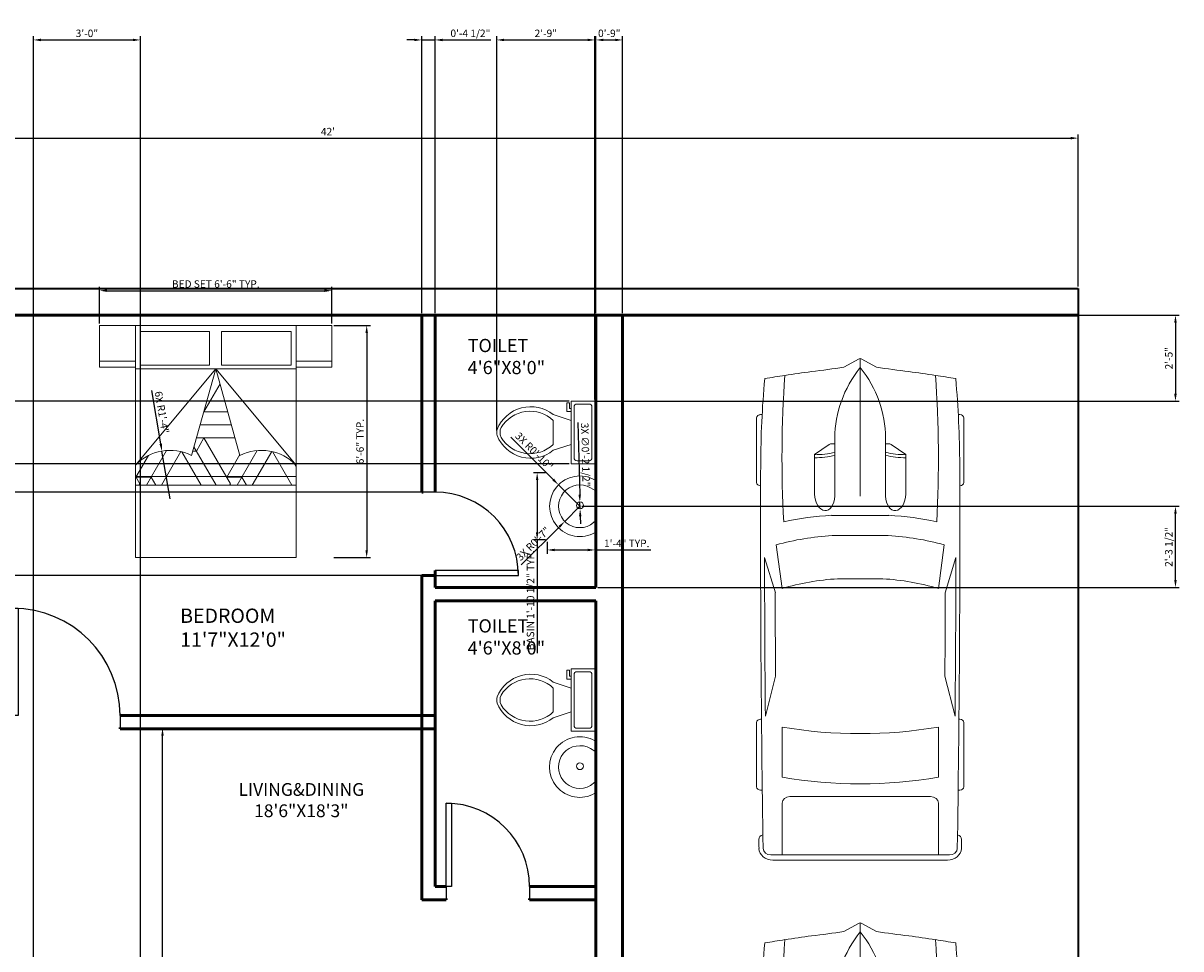
# Model space of a CAD drawing. Units: inches. Extents: x 1455 to 2044, y 1728 to 2439.
# Tile 4 of 4: x 1655 to 2044, y 2128 to 2439. Entities that reach past the tile are written whole.
import ezdxf

# ---------------------------------------------------------------- set-up
doc = ezdxf.new("R2010")
doc.units = ezdxf.units.IN
for name, color, linetype, lineweight in [('A-ANNO-DIMS', 2, 'Continuous', 18), ('A-AREA-IDEN', 7, 'Continuous', 25), ('A-DOOR', 4, 'Continuous', 25), ('A-FLOR-FIXT', 9, 'Continuous', 18), ('A-FURN', 8, 'Continuous', 18), ('A-WALL', 7, 'Continuous', 50), ('C-PRKG-VEHI', 8, 'Continuous', 13), ('C-PROP', 7, 'Continuous', 35)]:
    doc.layers.add(name, color=color, linetype=linetype, lineweight=lineweight)
doc.styles.get("Standard").update_dxf_attribs({"font": 'arial.ttf'})
doc.dimstyles.new('ISO-25', dxfattribs={"dimtxt": 2.5, "dimasz": 2.5, "dimexe": 1.25, "dimexo": 0.625, "dimtad": 1, "dimlunit": 3, "dimtxsty": 'Standard', "dimcen": 2.5, "dimadec": 0, "dimazin": 0, "dimtfac": 1, "dimtmove": 0, "dimatfit": 3, "dimfxl": 1, "dimarcsym": 0})

# ---------------------------------------------------------------- blocks, each defined once
blk = doc.blocks.new('*U7')
for p, q in [((0, 0), (0, -4)), ((36, 0), (36, -4))]:
    blk.add_line(p, q)
blk.add_lwpolyline([(0, 0), (0, 36), (1.75, 36), (1.75, 0)], close=True)
blk.add_arc((0, 0), 36, 0, 90)
blk = doc.blocks.new('*U4')
for p, q in [((-28, 0), (-28, -4)), ((0, 0), (0, -4))]:
    blk.add_line(p, q)
blk.add_lwpolyline([(0, 0), (0, 28), (-1.75, 28), (-1.75, 0)], close=True)
blk.add_arc((0, 0), 28, 90, 180)
blk = doc.blocks.new('*U5')
for p, q in [((0, 0), (0, -4)), ((28, 0), (28, -4))]:
    blk.add_line(p, q)
blk.add_lwpolyline([(0, 0), (0, 28), (1.75, 28), (1.75, 0)], close=True)
blk.add_arc((0, 0), 28, 0, 90)
blk = doc.blocks.new('*U2')
for p, q in [((9.5, -6), (9.5, -2)), ((-10, -8.5), (-8, -8.5)), ((-10, -9.5), (-10, -8.5)), ((-7, -9.5), (-10, -9.5)), ((-8, -8.5), (-8, -8)), ((-7, -8), (-7, -9.5)), ((-4, -8), (-6, -14)), ((4, -8), (6, -14)), ((4, -14), (-4, -14))]:
    blk.add_line(p, q)
blk.add_lwpolyline([(10.5, -8), (10.5, 0), (-10.5, 0), (-10.5, -8)], close=True)
for points in [[(-9.5, -2), (-9.5, -6)], [(8.5, -1), (-8.5, -1)], [(-8.5, -7), (8.5, -7)]]:
    blk.add_lwpolyline(points)
for centre, radius, start, end in [((-8.62, -1.88), 0.884, 81.8699, 188.1301), ((8.62, -1.88), 0.884, 351.8699, 98.1301), ((-8.62, -6.12), 0.884, 171.8699, 278.1301), ((8.62, -6.12), 0.884, 261.8699, 8.1301), ((3.52, -21.58), 12.17, 141.4691, 247.9714), ((4.2, -21.82), 11.33, 136.3677, 238.9468), ((-3.52, -21.58), 12.17, 292.0284, 38.5307), ((-4.2, -21.82), 11.33, 301.053, 43.6321), ((0, -27.88), 4, 245.7318, 294.2682), ((0, -29), 4, 254.8605, 285.1395)]:
    blk.add_arc(centre, radius, start, end)
blk = doc.blocks.new('*D17')
at = {"layer": 'A-ANNO-DIMS', "color": 0, "lineweight": -2, "transparency": 16777216}
for p, q in [((1505.58, 2350.2), (1505.58, 2401.3)), ((1508.08, 2400.05), (2007.08, 2400.05)), ((2009.58, 2350.2), (2009.58, 2401.3))]:
    blk.add_line(p, q, dxfattribs=at)
at = {"layer": 'A-ANNO-DIMS', "color": 0, "transparency": 16777216}
for points in [[(1508.08, 2400.47), (1508.08, 2399.63), (1505.58, 2400.05)], [(2007.08, 2400.47), (2007.08, 2399.63), (2009.58, 2400.05)]]:
    blk.add_solid(points, dxfattribs=at)
at = {"layer": 'Defpoints', "color": 0, "transparency": 16777216}
for p in [(2009.58, 2400.05), (1505.58, 2349.58), (2009.58, 2349.58)]:
    blk.add_point(p, dxfattribs=at)
at = {"layer": 'A-ANNO-DIMS', "color": 0, "transparency": 16777216, "insert": (1757.58, 2401.93), "char_height": 2.5, "attachment_point": 5}
blk.add_mtext("42'", dxfattribs=at)
blk = doc.blocks.new('*U19')
for p, q in [((21.1, 37.41), (21.1, 36.83)), ((46.55, 38.89), (22.35, 38.89)), ((47.8, 37.39), (47.8, 37.41)), ((87.99, 31.87), (74.76, 35.92)), ((134.31, 35.6), (119.29, 31.78)), ((135.45, 37.07), (135.45, 37.41)), ((136.7, 38.89), (160.9, 38.89)), ((162.15, 37.41), (162.15, 36.77)), ((70.03, 31.54), (86.41, 29.35)), ((186.47, -33.5), (186.47, 33.5)), ((188.4, -32.76), (188.4, 32.76)), ((138.42, 29.35), (157.25, 29.35)), ((164.52, 26.39), (164.52, -26.39)), ((186.47, 29.35), (167.01, 29.35)), ((32.27, 11.63), (36.13, 17.17)), ((36.13, 17.17), (50.94, 17.17)), ((29.77, 9.51), (51.68, 9.51)), ((32.12, 9.51), (32.12, 11.15)), ((58.92, -10.77), (58.92, 10.77)), ((66.55, -10.53), (66.55, 10.53)), ((186.47, -10.53), (186.47, 10.53)), ((3.27, 6.13), (0.1, 0.41)), ((82.74, 8.5), (82.74, -8.5)), ((0, 0), (51.68, 0)), ((0.1, -0.41), (3.27, -6.13)), ((29.77, -9.51), (51.68, -9.51)), ((32.12, -9.51), (32.12, -11.15)), ((32.27, -11.63), (36.13, -17.17)), ((36.13, -17.17), (50.94, -17.17)), ((86.41, -29.35), (70.03, -31.54)), ((157.25, -29.35), (138.42, -29.35)), ((167.01, -29.35), (186.47, -29.35)), ((87.99, -31.87), (74.76, -35.92)), ((134.31, -35.6), (119.29, -31.78)), ((21.1, -37.41), (21.1, -36.83)), ((46.55, -38.89), (22.35, -38.89)), ((47.8, -37.39), (47.8, -37.41)), ((135.45, -37.07), (135.45, -37.41)), ((136.7, -38.89), (160.9, -38.89)), ((162.15, -37.41), (162.15, -36.77))]:
    blk.add_line(p, q)
for centre, major_axis, ratio, start_param, end_param in [((266.03, -27.52), (0, 313.31), 0.842304, 1.367076, 1.39176), ((41.19, -490.86), (0, 528.23), 0.842304, 0.00281, 0.075598), ((22.35, 37.41), (0, -1.48), 0.842304, 3.141593, 4.712389), ((64.48, -10555.62), (0, 10593.03), 0.842304, -0.013397, 0.002797), ((46.55, 37.41), (0, 1.48), 0.842304, -1.570796, 0), ((64.48, -10555.62), (0, -10591.55), 0.842304, 3.133765, 3.140441), ((136.7, 37.41), (0, -1.48), 0.842304, 3.141593, 4.712389), ((160.9, 37.41), (0, 1.48), 0.842304, -1.570796, 0), ((180.63, 35.84), (0, 2.22), 0.842304, -0.013017, 1.249894), ((64.48, -10556.36), (0, 10595.31), 0.842304, -0.013397, -0.013017), ((183.98, 33.5), (0, -2.96), 0.842304, 1.570796, 3.128196), ((183.98, 32.76), (0, -5.25), 0.842304, 1.570796, 3.128196), ((135.29, 5.39), (0, 81.77), 0.842304, 1.245306, 1.50788), ((95.79, -3666.35), (0, -3698.24), 0.842304, 3.134049, 3.144098), ((259.18, -27.52), (0, -305.3), 0.842304, 4.528606, 4.561838), ((37.47, -593.96), (0, -623.33), 0.842304, 3.096046, 3.200911), ((134.4, 5.39), (0, -89.78), 0.842304, 4.449482, 4.652344), ((149.6, 2.8), (0, -79.58), 0.842304, 4.372215, 4.640744), ((17.08, 0), (0, 147.02), 0.842304, 4.511394, 4.913384), ((35.91, 0), (0, 147.02), 0.842304, 4.511394, 4.913384), ((167.01, 26.39), (0, 2.96), 0.842304, 0, 1.570796), ((-204.49, 52.4), (0, -250.96), 0.842304, 1.385369, 1.434372), ((13.04, 17.01), (0, 27.42), 0.842304, 4.435146, 4.718221), ((14.2, 17.01), (0, 27.42), 0.842304, 4.435146, 4.718221), ((50.79, 13.34), (6.34, -0.36), 0.603834, -1.395552, 1.581315), ((29.77, -46.66), (0, 56.17), 0.842304, 0, 0.590319), ((32.75, 11.15), (0, 0.74), 0.842304, 0.879714, 1.570796), ((0.62, 0), (0, -0.74), 0.842304, 4.131459, 5.293319), ((29.77, 46.66), (0, 56.17), 0.842304, 2.551274, 3.141593), ((-204.49, -52.4), (0, 250.96), 0.842304, -1.434372, -1.385369), ((149.6, -2.8), (0, -79.58), 0.842304, -1.499151, -1.230623), ((32.75, -11.15), (0, -0.74), 0.842304, 4.712389, 5.403472), ((13.04, -17.01), (0, -27.42), 0.842304, 1.564964, 1.848039), ((14.2, -17.01), (0, -27.42), 0.842304, 1.564964, 1.848039), ((134.4, -5.39), (0, -89.78), 0.842304, -1.510751, -1.307889), ((135.29, -5.39), (0, -81.77), 0.842304, -1.50788, -1.245306), ((259.18, 27.52), (0, 305.3), 0.842304, 1.721348, 1.754579), ((266.03, 27.52), (0, 313.31), 0.842304, 1.749832, 1.774517), ((37.47, 593.96), (0, -623.33), 0.842304, -0.059319, 0.045547), ((167.01, -26.39), (0, -2.96), 0.842304, 4.712389, 6.283185), ((95.79, 3666.35), (0, -3698.24), 0.842304, -0.002505, 0.007544), ((183.98, -33.5), (0, 2.96), 0.842304, 3.15499, 4.712389), ((183.98, -32.76), (0, -5.25), 0.842304, 0.013397, 1.570796), ((41.19, 490.86), (0, -528.23), 0.842304, -0.075598, -0.00281), ((22.35, -37.41), (0, 1.48), 0.842304, 1.570796, 3.141593), ((64.48, 10555.62), (0, 10593.03), 0.842304, 3.138796, 3.15499), ((46.55, -37.41), (0, -1.48), 0.842304, 0, 1.570796), ((64.48, 10555.62), (0, -10591.55), 0.842304, 0.001152, 0.007828), ((136.7, -37.41), (0, -1.48), 0.842304, -1.570796, 0), ((160.9, -37.41), (0, 1.48), 0.842304, 3.141593, 4.712389), ((180.63, -35.84), (0, -2.22), 0.842304, -1.249894, 0.013017), ((64.48, 10556.36), (0, 10595.31), 0.842304, 3.15461, 3.15499)]:
    blk.add_ellipse(centre, major_axis=major_axis, ratio=ratio, start_param=start_param, end_param=end_param)
at = {"extrusion": (0, 0, -1)}
blk.add_ellipse((50.79, -13.34), major_axis=(6.34, 0.36), ratio=0.603834, start_param=-1.395552, end_param=1.581315, dxfattribs=at)
blk = doc.blocks.new('*D20')
at = {"layer": 'A-ANNO-DIMS', "color": 0, "lineweight": -2, "transparency": 16777216}
for p, q in [((1702.63, 2201.77), (1703.25, 2201.77)), ((1702, 1985.27), (1702, 2199.27)), ((1702.63, 1982.77), (1703.25, 1982.77))]:
    blk.add_line(p, q, dxfattribs=at)
at = {"layer": 'A-ANNO-DIMS', "color": 0, "transparency": 16777216}
for points in [[(1701.59, 2199.27), (1702.42, 2199.27), (1702, 2201.77)], [(1701.59, 1985.27), (1702.42, 1985.27), (1702, 1982.77)]]:
    blk.add_solid(points, dxfattribs=at)
at = {"layer": 'Defpoints', "color": 0, "transparency": 16777216}
for p in [(1702, 2201.77), (1702, 2201.77), (1702, 1982.77)]:
    blk.add_point(p, dxfattribs=at)
at = {"layer": 'A-ANNO-DIMS', "color": 0, "transparency": 16777216, "insert": (1700.1, 2092.27), "char_height": 2.5, "attachment_point": 5, "rotation": 90}
blk.add_mtext('18\'-3"', dxfattribs=at)
blk = doc.blocks.new('BED-DOUBLE-WITH-NIGHTSTANDS')
h = blk.add_hatch()
h.set_pattern_fill('ESCHER', color=256, angle=-270)
h.set_pattern_definition([(150, (2210.078, -2055.985), (7e-09, -30.48), [27.94, -2.54]), (270, (2210.078, -2055.985), (26.39645, 15.24), [27.94, -2.54]), (30, (2210.078, -2055.985), (7e-09, 30.48), [27.94, -2.54]), (150, (2210.078, -2053.445), (7e-09, -30.48), [5.08, -25.4]), (30, (2210.078, -2053.445), (7e-09, 30.48), [5.08, -25.4]), (150, (2207.88, -2057.255), (7e-09, -30.48), [5.08, -25.4]), (270, (2207.88, -2057.255), (26.39645, 15.24), [5.08, -25.4]), (30, (2212.278, -2057.255), (7e-09, 30.48), [5.08, -25.4]), (270, (2212.278, -2057.255), (26.39645, 15.24), [5.08, -25.4]), (150, (2210.078, -2066.145), (7e-09, -30.48), [5.08, -25.4]), (30, (2210.078, -2066.145), (7e-09, 30.48), [5.08, -25.4]), (150, (2218.877, -2050.905), (7e-09, -30.48), [5.08, -25.4]), (270, (2218.877, -2050.905), (26.39645, 15.24), [5.08, -25.4]), (30, (2201.28, -2050.905), (7e-09, 30.48), [5.08, -25.4]), (270, (2201.28, -2050.905), (26.39645, 15.24), [5.08, -25.4]), (90, (2205.68, -2050.905), (-26.39645, -15.24), [17.78, -12.7]), (90, (2214.478, -2050.905), (-26.39645, -15.24), [17.78, -12.7]), (210, (2203.48, -2054.715), (-7e-09, -30.48), [17.78, -12.7]), (210, (2207.88, -2062.335), (-7e-09, -30.48), [17.78, -12.7]), (330, (2212.278, -2062.335), (26.39645, 15.24), [17.78, -12.7]), (330, (2216.678, -2054.715), (26.39645, 15.24), [17.78, -12.7])])
h.paths.add_polyline_path([(-31.09, 54, 0.326433), (-34.36, 35.12), (-63.46, 27), (-34.36, 18.88, 0.326433), (-31.09, 0), (-27.21, 0), (-27.21, 54)])
h.paths.add_polyline_path([(-27.21, 54), (-27.21, 0), (-24.3, 0), (-24.3, 54)])
for p, q in [((-78, 54), (-78, 66)), ((-78, 66), (-66, 66)), ((-66, 66), (-66, 54)), ((-66, 66), (-64, 66)), ((-64, 66), (-64, 54)), ((-63.46, 0), (-63.46, 54)), ((-63.46, 27), (-31.09, 54)), ((-63.46, 27), (-34.36, 35.12)), ((-76.01, 28.95), (-64.69, 28.95)), ((-76.01, 24.95), (-64.69, 24.95)), ((-63.46, 27), (-31.09, 0)), ((-63.46, 27), (-34.36, 18.88)), ((-78, 0), (-78, -12)), ((-66, -12), (-66, 0)), ((-64, -12), (-64, 0)), ((-78, -12), (-66, -12)), ((-66, -12), (-64, -12))]:
    blk.add_line(p, q)
for points in [[(0, 0), (0, 54), (-78, 54), (-78, 0)], [(-27.21, 0), (-27.21, 54), (-24.3, 54), (-24.3, 0)]]:
    blk.add_lwpolyline(points, close=True)
for points in [[(-76.01, 28.95), (-76.01, 52.28), (-64.69, 52.28), (-64.69, 28.95)], [(-64.69, 24.95), (-64.69, 1.63), (-76.01, 1.63), (-76.01, 24.95)]]:
    blk.add_lwpolyline(points)
for centre, start, end in [((-19.81, 42.32), 134.0109, 206.3245), ((-19.81, 11.68), 153.6755, 225.9891)]:
    blk.add_arc(centre, 16.24, start, end)
blk = doc.blocks.new('BASIN-WALL-MOUNT')
for p, q in [((-6.21, 3.6), (-5.3, 5.1)), ((6.21, 3.6), (5.05, 5.1))]:
    blk.add_line(p, q)
blk.add_circle((-0.29, 0.03), 1.16)
for radius in [10.18, 7.18]:
    blk.add_arc((0, 0), radius, 149.9376, 30.0624)
blk = doc.blocks.new('*D23')
at = {"layer": 'A-ANNO-DIMS', "color": 0, "lineweight": -2, "transparency": 16777216}
for p, q in [((1680.89, 2337.73), (1680.89, 2350.05)), ((1758.89, 2337.73), (1758.89, 2350.05)), ((1683.39, 2348.8), (1756.39, 2348.8))]:
    blk.add_line(p, q, dxfattribs=at)
at = {"layer": 'A-ANNO-DIMS', "color": 0, "transparency": 16777216}
for points in [[(1683.39, 2349.22), (1683.39, 2348.39), (1680.89, 2348.8)], [(1756.39, 2349.22), (1756.39, 2348.39), (1758.89, 2348.8)]]:
    blk.add_solid(points, dxfattribs=at)
at = {"layer": 'Defpoints', "color": 0, "transparency": 16777216}
for p in [(1758.89, 2348.8), (1680.89, 2337.1), (1758.89, 2337.1)]:
    blk.add_point(p, dxfattribs=at)
at = {"layer": 'A-ANNO-DIMS', "color": 0, "transparency": 16777216, "insert": (1719.89, 2350.72), "char_height": 2.5, "attachment_point": 5}
blk.add_mtext('BED SET 6\'-6" TYP.', dxfattribs=at)
blk = doc.blocks.new('*D24')
at = {"layer": 'A-ANNO-DIMS', "color": 0, "lineweight": -2, "transparency": 16777216}
for p, q in [((1759.51, 2337.1), (1771.84, 2337.1)), ((1770.59, 2334.6), (1770.59, 2261.6)), ((1759.51, 2259.1), (1771.84, 2259.1))]:
    blk.add_line(p, q, dxfattribs=at)
at = {"layer": 'A-ANNO-DIMS', "color": 0, "transparency": 16777216}
for points in [[(1770.17, 2334.6), (1771.01, 2334.6), (1770.59, 2337.1)], [(1770.17, 2261.6), (1771.01, 2261.6), (1770.59, 2259.1)]]:
    blk.add_solid(points, dxfattribs=at)
at = {"layer": 'Defpoints', "color": 0, "transparency": 16777216}
for p in [(1758.89, 2337.1), (1758.89, 2259.1), (1770.59, 2259.1)]:
    blk.add_point(p, dxfattribs=at)
at = {"layer": 'A-ANNO-DIMS', "color": 0, "transparency": 16777216, "insert": (1768.69, 2298.1), "char_height": 2.5, "attachment_point": 5, "rotation": 90}
blk.add_mtext('6\'-6" TYP.', dxfattribs=at)
blk = doc.blocks.new('*D25')
at = {"layer": 'A-ANNO-DIMS', "color": 0, "lineweight": -2, "transparency": 16777216}
for p, q in [((1830.62, 2287.65), (1826.61, 2287.65)), ((1827.86, 2285.15), (1827.86, 2267.57)), ((1830.62, 2265.07), (1826.61, 2265.07)), ((1827.86, 2265.07), (1827.86, 2226.98))]:
    blk.add_line(p, q, dxfattribs=at)
at = {"layer": 'A-ANNO-DIMS', "color": 0, "transparency": 16777216}
for points in [[(1827.44, 2285.15), (1828.27, 2285.15), (1827.86, 2287.65)], [(1827.44, 2267.57), (1828.27, 2267.57), (1827.86, 2265.07)]]:
    blk.add_solid(points, dxfattribs=at)
at = {"layer": 'Defpoints', "color": 0, "transparency": 16777216}
for p in [(1831.24, 2287.65), (1827.86, 2265.07), (1831.24, 2265.07)]:
    blk.add_point(p, dxfattribs=at)
at = {"layer": 'A-ANNO-DIMS', "color": 0, "transparency": 16777216, "insert": (1825.94, 2244.78), "char_height": 2.5, "attachment_point": 5, "rotation": 90}
blk.add_mtext('BASIN 1\'-10 1/2" TYP.', dxfattribs=at)
blk = doc.blocks.new('*D26')
at = {"layer": 'A-ANNO-DIMS', "color": 0, "lineweight": -2, "transparency": 16777216}
for p, q in [((1831.24, 2264.45), (1831.24, 2260.44)), ((1847.32, 2264.45), (1847.32, 2260.44)), ((1833.74, 2261.69), (1844.82, 2261.69)), ((1847.32, 2261.69), (1866.07, 2261.69))]:
    blk.add_line(p, q, dxfattribs=at)
at = {"layer": 'A-ANNO-DIMS', "color": 0, "transparency": 16777216}
for points in [[(1833.74, 2262.1), (1833.74, 2261.27), (1831.24, 2261.69)], [(1844.82, 2262.1), (1844.82, 2261.27), (1847.32, 2261.69)]]:
    blk.add_solid(points, dxfattribs=at)
at = {"layer": 'Defpoints', "color": 0, "transparency": 16777216}
for p in [(1831.24, 2265.07), (1847.32, 2265.07), (1847.32, 2261.69)]:
    blk.add_point(p, dxfattribs=at)
at = {"layer": 'A-ANNO-DIMS', "color": 0, "transparency": 16777216, "insert": (1857.94, 2263.57), "char_height": 2.5, "attachment_point": 5}
blk.add_mtext('1\'-4" TYP.', dxfattribs=at)
blk = doc.blocks.new('*D32')
at = {"layer": 'A-ANNO-DIMS', "color": 0, "lineweight": -2, "transparency": 16777216}
for p, q in [((1658.63, 2034.7), (1658.63, 2434.3)), ((1661.13, 2433.05), (1692.08, 2433.05)), ((1694.58, 2034.7), (1694.58, 2434.3))]:
    blk.add_line(p, q, dxfattribs=at)
at = {"layer": 'A-ANNO-DIMS', "color": 0, "transparency": 16777216}
for points in [[(1661.13, 2433.46), (1661.13, 2432.63), (1658.63, 2433.05)], [(1692.08, 2433.46), (1692.08, 2432.63), (1694.58, 2433.05)]]:
    blk.add_solid(points, dxfattribs=at)
at = {"layer": 'Defpoints', "color": 0, "transparency": 16777216}
for p in [(1694.58, 2433.05), (1658.63, 2034.08), (1694.58, 2034.08)]:
    blk.add_point(p, dxfattribs=at)
at = {"layer": 'A-ANNO-DIMS', "color": 0, "transparency": 16777216, "insert": (1676.61, 2434.95), "char_height": 2.5, "attachment_point": 5}
blk.add_mtext('3\'-0"', dxfattribs=at)
blk = doc.blocks.new('*D37')
at = {"layer": 'A-ANNO-DIMS', "color": 0, "lineweight": -2, "transparency": 16777216}
for p, q in [((1792.95, 2281.09), (1471.63, 2281.09)), ((1472.88, 2255.58), (1472.88, 2278.59)), ((1792.95, 2253.08), (1471.63, 2253.08))]:
    blk.add_line(p, q, dxfattribs=at)
at = {"layer": 'A-ANNO-DIMS', "color": 0, "transparency": 16777216}
for points in [[(1472.46, 2278.59), (1473.3, 2278.59), (1472.88, 2281.09)], [(1472.46, 2255.58), (1473.3, 2255.58), (1472.88, 2253.08)]]:
    blk.add_solid(points, dxfattribs=at)
at = {"layer": 'Defpoints', "color": 0, "transparency": 16777216}
for p in [(1472.88, 2281.09), (1793.58, 2281.09), (1793.58, 2253.08)]:
    blk.add_point(p, dxfattribs=at)
at = {"layer": 'A-ANNO-DIMS', "color": 0, "transparency": 16777216, "insert": (1471, 2267.09), "char_height": 2.5, "attachment_point": 5, "rotation": 90}
blk.add_mtext('2\'-4"', dxfattribs=at)
blk = doc.blocks.new('*D38')
at = {"layer": 'A-ANNO-DIMS', "color": 0, "lineweight": -2, "transparency": 16777216}
for p, q in [((1842.84, 2276.36), (2043.53, 2276.36)), ((2042.28, 2251.58), (2042.28, 2273.86)), ((1848.2, 2249.08), (2043.53, 2249.08))]:
    blk.add_line(p, q, dxfattribs=at)
at = {"layer": 'A-ANNO-DIMS', "color": 0, "transparency": 16777216}
for points in [[(2041.86, 2273.86), (2042.7, 2273.86), (2042.28, 2276.36)], [(2041.86, 2251.58), (2042.7, 2251.58), (2042.28, 2249.08)]]:
    blk.add_solid(points, dxfattribs=at)
at = {"layer": 'Defpoints', "color": 0, "transparency": 16777216}
for p in [(1842.22, 2276.36), (2042.28, 2276.36), (1847.58, 2249.08)]:
    blk.add_point(p, dxfattribs=at)
at = {"layer": 'A-ANNO-DIMS', "color": 0, "transparency": 16777216, "insert": (2040.36, 2262.72), "char_height": 2.5, "attachment_point": 5, "rotation": 90}
blk.add_mtext('2\'-3 1/2"', dxfattribs=at)
blk = doc.blocks.new('*D39')
at = {"layer": 'A-ANNO-DIMS', "color": 0, "lineweight": -2, "transparency": 16777216}
for p, q in [((1848.2, 2340.58), (2043.53, 2340.58)), ((2042.28, 2338.08), (2042.28, 2314.16)), ((1847.9, 2311.66), (2043.53, 2311.66))]:
    blk.add_line(p, q, dxfattribs=at)
at = {"layer": 'A-ANNO-DIMS', "color": 0, "transparency": 16777216}
for points in [[(2041.86, 2338.08), (2042.7, 2338.08), (2042.28, 2340.58)], [(2041.86, 2314.16), (2042.7, 2314.16), (2042.28, 2311.66)]]:
    blk.add_solid(points, dxfattribs=at)
at = {"layer": 'Defpoints', "color": 0, "transparency": 16777216}
for p in [(1847.58, 2340.58), (1847.27, 2311.66), (2042.28, 2311.66)]:
    blk.add_point(p, dxfattribs=at)
at = {"layer": 'A-ANNO-DIMS', "color": 0, "transparency": 16777216, "insert": (2040.38, 2326.12), "char_height": 2.5, "attachment_point": 5, "rotation": 90}
blk.add_mtext('2\'-5"', dxfattribs=at)
blk = doc.blocks.new('*D40')
at = {"layer": 'A-ANNO-DIMS', "color": 0, "lineweight": -2, "transparency": 16777216}
for p, q in [((1847.58, 2341.2), (1847.58, 2434.3)), ((1850.08, 2433.05), (1854.08, 2433.05)), ((1856.58, 2341.2), (1856.58, 2434.3))]:
    blk.add_line(p, q, dxfattribs=at)
at = {"layer": 'A-ANNO-DIMS', "color": 0, "transparency": 16777216}
for points in [[(1850.08, 2433.46), (1850.08, 2432.63), (1847.58, 2433.05)], [(1854.08, 2433.46), (1854.08, 2432.63), (1856.58, 2433.05)]]:
    blk.add_solid(points, dxfattribs=at)
at = {"layer": 'Defpoints', "color": 0, "transparency": 16777216}
for p in [(1856.58, 2433.05), (1847.58, 2340.58), (1856.58, 2340.58)]:
    blk.add_point(p, dxfattribs=at)
at = {"layer": 'A-ANNO-DIMS', "color": 0, "transparency": 16777216, "insert": (1852.08, 2434.95), "char_height": 2.5, "attachment_point": 5}
blk.add_mtext('0\'-9"', dxfattribs=at)
blk = doc.blocks.new('*D41')
at = {"layer": 'A-ANNO-DIMS', "color": 0, "lineweight": -2, "transparency": 16777216}
for p, q in [((1786.58, 2433.05), (1784.08, 2433.05)), ((1789.08, 2341.2), (1789.08, 2434.3)), ((1789.08, 2433.05), (1793.58, 2433.05)), ((1793.58, 2341.2), (1793.58, 2434.3)), ((1796.08, 2433.05), (1812.3, 2433.05))]:
    blk.add_line(p, q, dxfattribs=at)
at = {"layer": 'A-ANNO-DIMS', "color": 0, "transparency": 16777216}
for points in [[(1786.58, 2433.46), (1786.58, 2432.63), (1789.08, 2433.05)], [(1796.08, 2433.46), (1796.08, 2432.63), (1793.58, 2433.05)]]:
    blk.add_solid(points, dxfattribs=at)
at = {"layer": 'Defpoints', "color": 0, "transparency": 16777216}
for p in [(1793.58, 2433.05), (1789.08, 2340.58), (1793.58, 2340.58)]:
    blk.add_point(p, dxfattribs=at)
at = {"layer": 'A-ANNO-DIMS', "color": 0, "transparency": 16777216, "insert": (1805.44, 2434.96), "char_height": 2.5, "attachment_point": 5}
blk.add_mtext('0\'-4 1/2"', dxfattribs=at)
blk = doc.blocks.new('*D42')
at = {"layer": 'A-ANNO-DIMS', "color": 0, "lineweight": -2, "transparency": 16777216}
for p, q in [((1838.65, 2311.66), (1471.63, 2311.66)), ((1472.88, 2309.16), (1472.88, 2293.16)), ((1838.65, 2290.66), (1471.63, 2290.66))]:
    blk.add_line(p, q, dxfattribs=at)
at = {"layer": 'A-ANNO-DIMS', "color": 0, "transparency": 16777216}
for points in [[(1472.46, 2309.16), (1473.3, 2309.16), (1472.88, 2311.66)], [(1472.46, 2293.16), (1473.3, 2293.16), (1472.88, 2290.66)]]:
    blk.add_solid(points, dxfattribs=at)
at = {"layer": 'Defpoints', "color": 0, "transparency": 16777216}
for p in [(1839.27, 2311.66), (1472.88, 2290.66), (1839.27, 2290.66)]:
    blk.add_point(p, dxfattribs=at)
at = {"layer": 'A-ANNO-DIMS', "color": 0, "transparency": 16777216, "insert": (1470.98, 2301.16), "char_height": 2.5, "attachment_point": 5, "rotation": 90}
blk.add_mtext('1\'-9"', dxfattribs=at)
blk = doc.blocks.new('*D43')
at = {"layer": 'A-ANNO-DIMS', "color": 0, "lineweight": -2, "transparency": 16777216}
for p, q in [((1814.27, 2301.79), (1814.27, 2434.3)), ((1816.77, 2433.05), (1844.77, 2433.05)), ((1847.27, 2312.29), (1847.27, 2434.3))]:
    blk.add_line(p, q, dxfattribs=at)
at = {"layer": 'A-ANNO-DIMS', "color": 0, "transparency": 16777216}
for points in [[(1816.77, 2433.46), (1816.77, 2432.63), (1814.27, 2433.05)], [(1844.77, 2433.46), (1844.77, 2432.63), (1847.27, 2433.05)]]:
    blk.add_solid(points, dxfattribs=at)
at = {"layer": 'Defpoints', "color": 0, "transparency": 16777216}
for p in [(1847.27, 2433.05), (1847.27, 2311.66), (1814.27, 2301.16)]:
    blk.add_point(p, dxfattribs=at)
at = {"layer": 'A-ANNO-DIMS', "color": 0, "transparency": 16777216, "insert": (1830.77, 2434.95), "char_height": 2.5, "attachment_point": 5}
blk.add_mtext('2\'-9"', dxfattribs=at)
blk = doc.blocks.new('*D44')
at = {"layer": 'A-ANNO-DIMS', "color": 0, "lineweight": -2, "transparency": 16777216}
for p, q in [((1819.04, 2299.54), (1833.25, 2285.33)), ((1842.22, 2276.36), (1835.02, 2283.56))]:
    blk.add_line(p, q, dxfattribs=at)
at = {"layer": 'A-ANNO-DIMS', "color": 0, "transparency": 16777216}
blk.add_solid([(1833.55, 2285.62), (1832.96, 2285.03), (1835.02, 2283.56)], dxfattribs=at)
at = {"layer": 'Defpoints', "color": 0, "transparency": 16777216}
for p in [(1835.02, 2283.56), (1842.22, 2276.36)]:
    blk.add_point(p, dxfattribs=at)
at = {"layer": 'A-ANNO-DIMS', "color": 0, "transparency": 16777216, "insert": (1826.61, 2294.66), "char_height": 2.5, "attachment_point": 5, "rotation": 314.9851}
blk.add_mtext('3X R0\'-10"', dxfattribs=at)
blk = doc.blocks.new('*D45')
at = {"layer": 'A-ANNO-DIMS', "color": 0, "lineweight": -2, "transparency": 16777216}
for p, q in [((1842.22, 2276.36), (1837.14, 2271.28)), ((1822.54, 2256.67), (1835.37, 2269.51))]:
    blk.add_line(p, q, dxfattribs=at)
at = {"layer": 'A-ANNO-DIMS', "color": 0, "transparency": 16777216}
blk.add_solid([(1835.08, 2269.81), (1835.67, 2269.22), (1837.14, 2271.28)], dxfattribs=at)
at = {"layer": 'Defpoints', "color": 0, "transparency": 16777216}
for p in [(1842.22, 2276.36), (1837.14, 2271.28)]:
    blk.add_point(p, dxfattribs=at)
at = {"layer": 'A-ANNO-DIMS', "color": 0, "transparency": 16777216, "insert": (1826.73, 2263.55), "char_height": 2.5, "attachment_point": 5, "rotation": 45.0146}
blk.add_mtext('3X R0\'-7"', dxfattribs=at)
blk = doc.blocks.new('*D46')
at = {"layer": 'A-ANNO-DIMS', "color": 0, "lineweight": -2, "transparency": 16777216}
for p, q in [((1841.53, 2304.48), (1842.15, 2280.31)), ((1842.27, 2275.49), (1842.21, 2277.81)), ((1842.34, 2272.99), (1842.4, 2270.49))]:
    blk.add_line(p, q, dxfattribs=at)
at = {"layer": 'A-ANNO-DIMS', "color": 0, "transparency": 16777216}
for points in [[(1842.57, 2280.32), (1841.73, 2280.3), (1842.21, 2277.81)], [(1842.75, 2273), (1841.92, 2272.98), (1842.27, 2275.49)]]:
    blk.add_solid(points, dxfattribs=at)
at = {"layer": 'Defpoints', "color": 0, "transparency": 16777216}
for p in [(1842.21, 2277.81), (1842.27, 2275.49)]:
    blk.add_point(p, dxfattribs=at)
at = {"layer": 'A-ANNO-DIMS', "color": 0, "transparency": 16777216, "insert": (1843.78, 2293.69), "char_height": 2.5, "attachment_point": 5, "rotation": 271.46}
blk.add_mtext('3X ∅0\'-2 1/2"', dxfattribs=at)
blk = doc.blocks.new('*D47')
at = {"layer": 'A-ANNO-DIMS', "color": 0, "lineweight": -2, "transparency": 16777216}
for p, q in [((1698.27, 2315.28), (1701.37, 2297.38)), ((1704.57, 2278.91), (1701.8, 2294.91))]:
    blk.add_line(p, q, dxfattribs=at)
at = {"layer": 'A-ANNO-DIMS', "color": 0, "transparency": 16777216}
blk.add_solid([(1701.78, 2297.45), (1700.96, 2297.31), (1701.8, 2294.91)], dxfattribs=at)
at = {"layer": 'Defpoints', "color": 0, "transparency": 16777216}
for p in [(1701.8, 2294.91), (1704.57, 2278.91)]:
    blk.add_point(p, dxfattribs=at)
at = {"layer": 'A-ANNO-DIMS', "color": 0, "transparency": 16777216, "insert": (1701.48, 2307.89), "char_height": 2.5, "attachment_point": 5, "rotation": 279.8321}
blk.add_mtext('6X R1\'-4"', dxfattribs=at)

msp = doc.modelspace()

# ---------------------------------------------------------------- linework, layer by layer
at = {"layer": 'A-WALL'}
for p, q in [((1514.58, 2340.579), (2000.58, 2340.579)), ((1789.08, 2340.579), (1789.08, 2281.092)), ((1793.58, 2340.579), (1793.58, 2281.092)), ((1847.58, 2340.579), (1847.58, 2249.079)), ((1856.58, 2340.579), (1856.58, 1770.579)), ((1856.58, 2340.579), (2000.58, 2340.579)), ((2000.58, 2340.579), (2009.58, 2340.579)), ((1789.562, 2281.092), (1789.08, 2281.092)), ((1789.562, 2253.092), (1789.08, 2253.092)), ((1789.08, 2253.092), (1789.08, 2144.079)), ((1793.58, 2253.079), (1789.08, 2253.079)), ((1793.58, 2254.842), (1793.58, 2249.079)), ((1793.58, 2249.079), (1793.58, 2253.079)), ((1793.58, 2249.079), (1847.58, 2249.079)), ((1793.58, 2244.579), (1847.58, 2244.579)), ((1793.58, 2244.579), (1793.58, 2148.579)), ((1847.58, 2244.579), (1847.58, 1871.579)), ((1687.746, 2206.079), (1793.58, 2206.079)), ((1687.746, 2202.084), (1687.746, 2201.579)), ((1687.746, 2201.579), (1793.58, 2201.579)), ((1793.58, 2148.579), (1797.313, 2148.579)), ((1825.313, 2148.579), (1847.58, 2148.579)), ((1793.58, 2144.079), (1789.08, 2144.079)), ((1793.58, 2144.079), (1797.313, 2144.079)), ((1797.313, 2144.581), (1797.313, 2144.079)), ((1825.313, 2144.581), (1825.313, 2144.079)), ((1825.313, 2144.079), (1847.58, 2144.079))]:
    msp.add_line(p, q, dxfattribs=at)
at = {"layer": 'C-PROP'}
for p, q in [((1505.58, 2349.579), (2009.58, 2349.579)), ((2009.58, 2349.579), (2009.58, 1761.579))]:
    msp.add_line(p, q, dxfattribs=at)

# ---------------------------------------------------------------- block references
at = {"layer": 'A-DOOR', "rotation": 270}
msp.add_blockref('*U4', (1793.562, 2253.092), dxfattribs=at)
at = {"layer": 'A-DOOR'}
for name, p in [('*U7', (1651.746, 2206.084)), ('*U5', (1797.313, 2148.581))]:
    msp.add_blockref(name, p, dxfattribs=at)
at = {"layer": 'A-FLOR-FIXT'}
for name, p, rotation in [('*U2', (1847.271, 2301.165), 270), ('BASIN-WALL-MOUNT', (1842.217, 2276.359), 269.9999999999931), ('*U2', (1847.271, 2211.288), 270), ('BASIN-WALL-MOUNT', (1842.185, 2188.745), 269.9999999999931)]:
    msp.add_blockref(name, p, dxfattribs=dict(at, rotation=rotation))
at = {"layer": 'A-FURN', "rotation": 269.9999999999993}
msp.add_blockref('BED-DOUBLE-WITH-NIGHTSTANDS', (1692.89, 2259.104), dxfattribs=at)
at = {"layer": 'C-PRKG-VEHI', "xscale": 0.8946429665525277, "yscale": 0.8946429665525277, "zscale": 0.8946429665525277, "rotation": 270}
for p in [(1936.381, 2326.033), (1936.381, 2136.429)]:
    msp.add_blockref('*U19', p, dxfattribs=at)

# ---------------------------------------------------------------- texts
at = {"layer": 'A-AREA-IDEN', "attachment_point": 1}
for s, width, gutter_width, insert, char_height in [('TOILET\\P4\'6"X8\'0"', 39.57075, 22.204, (1804.513, 2332.603), 4.4408), ('BEDROOM\\P11\'7"X12\'0"', 85.70545, 24.072, (1707.939, 2241.987), 4.81444), ('TOILET\\P4\'6"X8\'0"', 39.57075, 22.204, (1804.513, 2238.39), 4.4408), ('LIVING&DINING\\P    18\'6"X18\'3"', 79.6794, 21.479, (1727.529, 2183.367), 4.29574)]:
    msp.add_mtext_dynamic_manual_height_columns(s, width=width, gutter_width=gutter_width, heights=[0], dxfattribs=dict(at, insert=insert, char_height=char_height))

# ---------------------------------------------------------------- dimensions: what is measured, and where the dimension line sits
at = {"layer": 'A-ANNO-DIMS'}
for base, p1, p2, override, picture, middle in [((1793.58, 2433.046), (1789.08, 2340.579), (1793.58, 2340.579), {"dimdec": 1, "dimlfac": 1, "dimrnd": 0, "dimzin": 1, "dimdsep": 46, "dimlunit": 4, "dimfrac": 2}, '*D41', (1805.44, 2434.964)), ((1694.58, 2433.046), (1658.632, 2034.079), (1694.58, 2034.079), {"dimdec": 1, "dimlfac": 1, "dimrnd": 0, "dimzin": 1, "dimdsep": 46, "dimlunit": 4, "dimfrac": 2}, '*D32', (1676.606, 2434.948)), ((1847.271, 2433.046), (1814.271, 2301.165), (1847.271, 2311.665), {"dimdec": 1, "dimlfac": 1, "dimrnd": 0, "dimzin": 1, "dimdsep": 46, "dimlunit": 4, "dimfrac": 2}, '*D43', (1830.771, 2434.947)), ((1856.58, 2433.046), (1847.58, 2340.579), (1856.58, 2340.579), {"dimdec": 1, "dimlfac": 1, "dimrnd": 0, "dimzin": 1, "dimdsep": 46, "dimlunit": 4, "dimfrac": 2}, '*D40', (1852.08, 2434.947)), ((2009.58, 2400.051), (1505.58, 2349.579), (2009.58, 2349.579), {"dimclrd": 0, "dimclre": 0, "dimclrt": 0}, '*D17', (1757.58, 2401.931))]:
    dim = msp.add_linear_dim(base=base, p1=p1, p2=p2, dimstyle='ISO-25', override=override, dxfattribs=at)
    dim.commit()
    dim.dimension.update_dxf_attribs({"geometry": picture, "text_midpoint": middle})
for base, p1, p2, text, picture, middle in [((1758.89, 2348.804), (1680.89, 2337.104), (1758.89, 2337.104), 'BED SET <> TYP.', '*D23', (1719.89, 2350.721)), ((1847.316, 2261.688), (1831.243, 2265.073), (1847.316, 2265.073), '<> TYP.', '*D26', (1857.943, 2263.569))]:
    dim = msp.add_linear_dim(base=base, p1=p1, p2=p2, text=text, dimstyle='ISO-25', override={"dimdec": 1, "dimlfac": 1, "dimrnd": 0, "dimzin": 1, "dimdsep": 46, "dimlunit": 4, "dimfrac": 2}, dxfattribs=at)
    dim.commit()
    dim.dimension.update_dxf_attribs({"geometry": picture, "text_midpoint": middle})
for base, p1, p2, override, picture, middle in [((2042.28, 2311.665), (1847.58, 2340.579), (1847.271, 2311.665), {"dimdec": 1, "dimlfac": 1, "dimrnd": 0, "dimzin": 1, "dimdsep": 46, "dimlunit": 4, "dimfrac": 2}, '*D39', (2040.378, 2326.122)), ((1472.88, 2290.665), (1839.271, 2311.665), (1839.271, 2290.665), {"dimdec": 1, "dimlfac": 1, "dimrnd": 0, "dimzin": 1, "dimdsep": 46, "dimlunit": 4, "dimfrac": 2}, '*D42', (1470.978, 2301.165)), ((1472.88, 2281.092), (1793.58, 2253.079), (1793.58, 2281.092), {"dimdec": 1, "dimlfac": 1, "dimrnd": 0, "dimzin": 1, "dimdsep": 46, "dimlunit": 4, "dimfrac": 2}, '*D37', (1470.999, 2267.086)), ((2042.28, 2276.359), (1847.58, 2249.079), (1842.217, 2276.359), {"dimdec": 1, "dimlfac": 1, "dimrnd": 0, "dimzin": 1, "dimdsep": 46, "dimlunit": 4, "dimfrac": 2}, '*D38', (2040.361, 2262.719)), ((1702.002, 2201.769), (1702.002, 1982.769), (1702.002, 2201.769), {"dimclrd": 0, "dimclre": 0, "dimclrt": 0}, '*D20', (1700.099, 2092.269))]:
    dim = msp.add_linear_dim(base=base, p1=p1, p2=p2, angle=90, dimstyle='ISO-25', override=override, dxfattribs=at)
    dim.commit()
    dim.dimension.update_dxf_attribs({"geometry": picture, "text_midpoint": middle})
for base, p1, p2, text, picture, middle in [((1770.59, 2259.104), (1758.89, 2337.104), (1758.89, 2259.104), '<> TYP.', '*D24', (1768.688, 2298.104)), ((1827.857, 2265.073), (1831.243, 2287.645), (1831.243, 2265.073), 'BASIN <> TYP.', '*D25', (1825.94, 2244.775))]:
    dim = msp.add_linear_dim(base=base, p1=p1, p2=p2, angle=270, text=text, dimstyle='ISO-25', override={"dimdec": 1, "dimlfac": 1, "dimrnd": 0, "dimzin": 1, "dimdsep": 46, "dimlunit": 4, "dimfrac": 2}, dxfattribs=at)
    dim.commit()
    dim.dimension.update_dxf_attribs({"geometry": picture, "text_midpoint": middle})
for center, mpoint, text, picture, middle in [((1704.569, 2278.913), (1701.796, 2294.914), '6X <>', '*D47', (1701.478, 2307.887)), ((1842.217, 2276.359), (1835.021, 2283.559), '3X <>', '*D44', (1826.611, 2294.665)), ((1842.217, 2276.359), (1837.142, 2271.282), '3X <>', '*D45', (1826.727, 2263.553))]:
    dim = msp.add_radius_dim(center=center, mpoint=mpoint, text=text, dimstyle='ISO-25', override={"dimdec": 1, "dimlfac": 1, "dimrnd": 0, "dimzin": 1, "dimdsep": 46, "dimlunit": 4, "dimfrac": 2}, dxfattribs=at)
    dim.commit()
    dim.dimension.update_dxf_attribs({"geometry": picture, "text_midpoint": middle})
dim = msp.add_diameter_dim_2p(p1=(1842.272, 2275.486), p2=(1842.213, 2277.807), text='3X <>', dimstyle='ISO-25', override={"dimdec": 1, "dimlfac": 1, "dimrnd": 0, "dimzin": 1, "dimdsep": 46, "dimlunit": 4, "dimfrac": 2}, dxfattribs=at)
dim.commit()
dim.dimension.update_dxf_attribs({"geometry": '*D46', "text_midpoint": (1841.809, 2293.641), "dimtype": 163})

doc.saveas('drawing.dxf')
